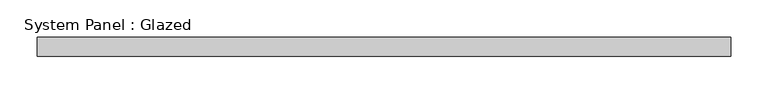
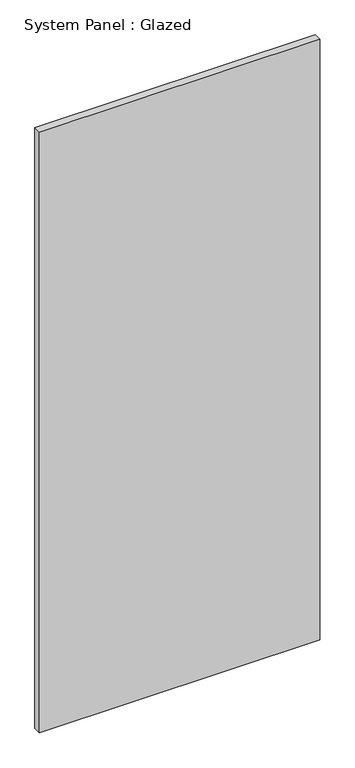
"""IFC4 building model written with IfcOpenShell, lengths in millimetres: plate geometry, System Panel : Glazed."""

from ifc_helpers import new_model, si_unit, origin, origin_with_axes, place, context, project, spatial, polyline, outline, extrude, source, transform, mapped, element, save


def system_panel_glazed_65c2c16a(model_context):
    return source(origin(), model_context, "Body", "SweptSolid", [
        extrude(outline(polyline([(463.95, 24.5), (-463.95, 24.5), (-463.95, 49.5), (463.95, 49.5), (463.95, 24.5)])), origin_with_axes(), (0.0, 0.0, 1.0), 2102.7143587),
    ])


if __name__ == "__main__":
    model = new_model("IFC4")
    model_context = context("Model", 3, world=origin())
    ifc_project = project(units=[si_unit("LENGTHUNIT", "METRE", prefix="MILLI")], contexts=[model_context])
    site = spatial("IfcSite", under=ifc_project)
    building = spatial("IfcBuilding", under=site)
    placement = place(None, origin())
    system_panel_glazed_shape = system_panel_glazed_65c2c16a(model_context)
    element("IfcPlate", 1, ObjectType="System Panel : Glazed", at=placement, inside=building, context=model_context, shape_type="MappedRepresentation", body=[
        mapped(system_panel_glazed_shape, transform((0.0, 0.0, 0.0), x_axis=(1.0, 0.0, 0.0), y_axis=(0.0, 1.0, 0.0), z_axis=(0.0, 0.0, 1.0))),
    ])
    save(model, "model.ifc")

# Revit data of these elements
# Type "System Panel : Glazed"
#   Keynote = "H11"
#   Construction Type Id = "GSP4R"
#   Analytic Construction = "1/8 in Pilkington single glazing"
#   Visual Light Transmittance = 0.9
#   Solar Heat Gain Coefficient = 0.86
#   Heat Transfer Coefficient (U) = 6.7069 W/(m²·K)
#   Define Thermal Properties by = 1
# Element 1 (IfcPlate, "System Panel : Glazed")
#   Materials on its faces: "Glass"
# Materials
#   "Glass": class "Glass", colour RGB 0 128 192, transparency 0.9, Description = "Soda Lime Glass", Cost = 0
